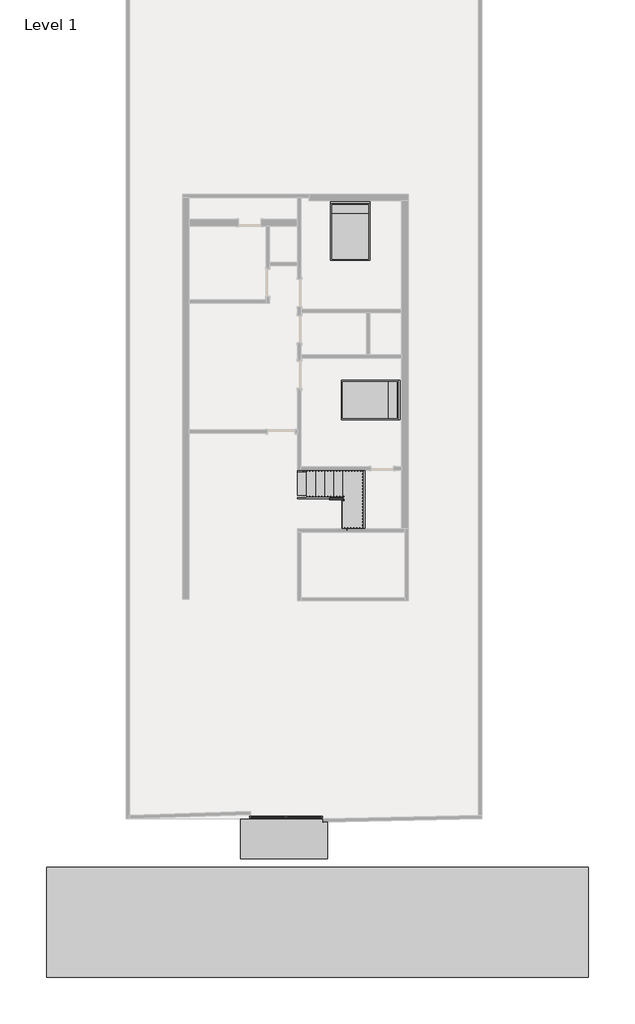
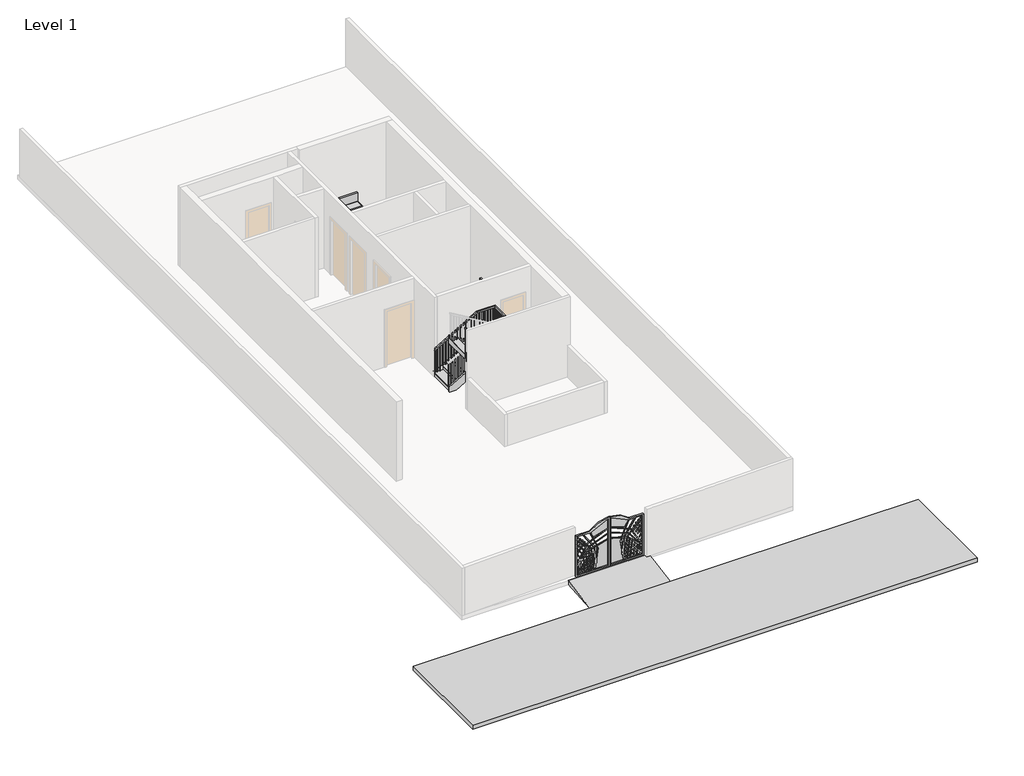
# One storey, part 2 of 2: 6 members, 3 proxies, 2 furniture elements, 1 railing, 1 stair flight.
"""IFC4 building model written with IfcOpenShell, lengths in millimetres."""

from ifc_helpers import new_model, si_unit, frame, origin, place, context, project, spatial, polyline, outline, extrude, faceted_brep, transform, mapped, element, save
from components import generic_models_6bc30956, generic_models_1_generic_models_1_3838245b, generic_models_2_generic_models_2_e98e430d, bed_17739_bed_17739_15c61121, stair_flight_ab8743af

model = new_model("IFC4")

# Units and contexts
model_context = context("Model", 3, world=origin())
ifc_project = project(units=[si_unit("LENGTHUNIT", "METRE", prefix="MILLI")], contexts=[model_context])

# Site, building, storey
site = spatial("IfcSite", under=ifc_project)
building = spatial("IfcBuilding", under=site)
storey = spatial("IfcBuildingStorey", under=building, Name="Level 1", Elevation=0.0)

# Proxies
placement = place(None, origin())
generic_models_shape = generic_models_6bc30956(model_context)
element("IfcBuildingElementProxy", 1, Name="Generic Models", at=placement, inside=storey, context=model_context, shape_type="MappedRepresentation", body=[
    mapped(generic_models_shape, transform((-1579.0915084, -13578.7130462, 0.0), x_axis=(1.0, 0.0, 0.0), y_axis=(0.0, 1.0, 0.0), z_axis=(0.0, 0.0, 1.0))),
])
generic_models_1_generic_models_1_shape = generic_models_1_generic_models_1_3838245b(model_context)
element("IfcBuildingElementProxy", 2, Name="Generic Models 1 : Generic Models 1", ObjectType="Generic Models 1 : Generic Models 1", at=placement, inside=storey, context=model_context, shape_type="MappedRepresentation", body=[
    mapped(generic_models_1_generic_models_1_shape, transform((0.0, 0.0, 0.0), x_axis=(1.0, 0.0, 0.0), y_axis=(0.0, 1.0, 0.0), z_axis=(0.0, 0.0, 1.0))),
])
generic_models_2_generic_models_2_shape = generic_models_2_generic_models_2_e98e430d(model_context)
element("IfcBuildingElementProxy", 3, Name="Generic Models 2 : Generic Models 2", ObjectType="Generic Models 2 : Generic Models 2", at=placement, inside=storey, context=model_context, shape_type="MappedRepresentation", body=[
    mapped(generic_models_2_generic_models_2_shape, transform((0.0, 0.0, 0.0), x_axis=(1.0, 0.0, 0.0), y_axis=(0.0, 1.0, 0.0), z_axis=(0.0, 0.0, 1.0))),
])

# Furniture
bed_17739_bed_17739_shape = bed_17739_bed_17739_15c61121(model_context)
element("IfcFurniture", 4, ObjectType="Bed_17739 : Bed_17739", at=placement, inside=storey, context=model_context, shape_type="MappedRepresentation", body=[
    mapped(bed_17739_bed_17739_shape, transform((592.6084916, 6126.1935985, 0.0), x_axis=(1.0, 0.0, 0.0), y_axis=(0.0, 1.0, 0.0), z_axis=(0.0, 0.0, 1.0))),
])
element("IfcFurniture", 5, ObjectType="Bed_17739 : Bed_17739", at=placement, inside=storey, context=model_context, shape_type="MappedRepresentation", body=[
    mapped(bed_17739_bed_17739_shape, transform((1259.3584916, 455.6435985, 0.0), x_axis=(0.0, -1.0, 0.0), y_axis=(1.0, 0.0, 0.0), z_axis=(0.0, 0.0, 1.0))),
])

# Members
element("IfcMember", 6, ObjectType="Stringer - 2\" Width", at=placement, inside=storey, context=model_context, shape_type="SweptSolid", body=[
    extrude(outline(polyline([(210.4752888, -1179.0415084), (0.0, -1179.0415084), (0.0, -935.6899318), (1151.9647059, 1022.6500682), (1151.9647059, 421.4905007), (210.4752888, -1179.0415084)])), frame((0.0, -1912.9064015, 0.0), z_axis=(0.0, 1.0, 0.0), x_axis=(0.0, 0.0, 1.0)), (0.0, 0.0, 1.0), 50.8),
])
element("IfcMember", 7, ObjectType="Stringer - 2\" Width", at=placement, inside=storey, context=model_context, shape_type="SweptSolid", body=[
    extrude(outline(polyline([(1043.4584916, -1862.1064015), (1094.2584916, -1862.1064015), (1094.2584916, -3894.1064015), (1043.4584916, -3894.1064015), (1043.4584916, -1862.1064015)])), frame((0.0, 0.0, 847.1647059), z_axis=(0.0, 0.0, 1.0), x_axis=(1.0, 0.0, 0.0)), (0.0, 0.0, 1.0), 304.8),
])
element("IfcMember", 8, ObjectType="Stringer - 2\" Width", at=placement, inside=storey, context=model_context, shape_type="SweptSolid", body=[
    extrude(outline(polyline([(847.1647059, 1091.3864826), (2182.7105829, -1179.0415084), (1829.0873079, -1179.0415084), (847.1647059, 490.2269151), (847.1647059, 1091.3864826)])), frame((0.0, -3944.9064015, 0.0), z_axis=(0.0, 1.0, 0.0), x_axis=(0.0, 0.0, 1.0)), (0.0, 0.0, 1.0), 50.8),
])
element("IfcMember", 9, ObjectType="Stringer - 2\" Width", at=placement, inside=storey, context=model_context, shape_type="SweptSolid", body=[
    extrude(outline(polyline([(210.4752888, -1179.0415084), (0.0, -1179.0415084), (0.0, -935.6899318), (723.4402491, 294.1584916), (1077.0635241, 294.1584916), (210.4752888, -1179.0415084)])), frame((0.0, -2878.1064015, 0.0), z_axis=(0.0, 1.0, 0.0), x_axis=(0.0, 0.0, 1.0)), (0.0, 0.0, 1.0), 50.8),
])
element("IfcMember", 10, ObjectType="Stringer - 2\" Width", at=placement, inside=storey, context=model_context, shape_type="SweptSolid", body=[
    extrude(outline(polyline([(294.1584916, -2827.3064015), (344.9584916, -2827.3064015), (344.9584916, -2852.7064015), (294.1584916, -2852.7064015), (294.1584916, -2827.3064015)])), frame((0.0, 0.0, 847.1647059), z_axis=(0.0, 0.0, 1.0), x_axis=(1.0, 0.0, 0.0)), (0.0, 0.0, 1.0), 304.8),
])
element("IfcMember", 11, ObjectType="Stringer - 2\" Width", at=placement, inside=storey, context=model_context, shape_type="SweptSolid", body=[
    extrude(outline(polyline([(932.6167197, 344.9584916), (1286.2399947, 344.9584916), (2182.7105829, -1179.0415084), (1829.0873079, -1179.0415084), (932.6167197, 344.9584916)])), frame((0.0, -2903.5064015, 0.0), z_axis=(0.0, 1.0, 0.0), x_axis=(0.0, 0.0, 1.0)), (0.0, 0.0, 1.0), 50.8),
])

# Railing
element("IfcRailing", 12, ObjectType="Handrail - Rectangular", at=placement, inside=storey, context=model_context, shape_type="SolidModel", body=[
    faceted_brep([(-1179.0415084, -1912.9064015, 1093.6941176), (-1179.0415084, -1912.9064015, 1034.7569051), (-1179.0415084, -1963.7064015, 1034.7569051), (-1179.0415084, -1963.7064015, 1093.6941176), (344.9584916, -1912.9064015, 1990.1647059), (358.7917529, -1912.9064015, 1939.3647059), (358.7917529, -1963.7064015, 1939.3647059), (344.9584916, -1963.7064015, 1990.1647059), (1043.4584916, -1912.9064015, 1990.1647059), (1043.4584916, -1912.9064015, 1939.3647059), (992.6584916, -1963.7064015, 1939.3647059), (992.6584916, -1963.7064015, 1990.1647059), (1043.4584916, -3894.1064015, 1990.1647059), (1043.4584916, -3894.1064015, 1939.3647059), (992.6584916, -3843.3064015, 1939.3647059), (992.6584916, -3843.3064015, 1990.1647059), (649.7584916, -3894.1064015, 1990.1647059), (635.9252304, -3894.1064015, 1939.3647059), (635.9252304, -3843.3064015, 1939.3647059), (649.7584916, -3843.3064015, 1990.1647059), (-1179.0415084, -3894.1064015, 3065.9294118), (-1179.0415084, -3843.3064015, 3065.9294118), (-1179.0415084, -3843.3064015, 3006.9921993), (-1179.0415084, -3894.1064015, 3006.9921993)], [[[0, 1, 2, 3]], [[1, 0, 4, 5]], [[2, 1, 5, 6]], [[3, 2, 6, 7]], [[0, 3, 7, 4]], [[5, 4, 8, 9]], [[6, 5, 9, 10]], [[7, 6, 10, 11]], [[4, 7, 11, 8]], [[9, 8, 12, 13]], [[10, 9, 13, 14]], [[11, 10, 14, 15]], [[8, 11, 15, 12]], [[13, 12, 16, 17]], [[14, 13, 17, 18]], [[15, 14, 18, 19]], [[12, 15, 19, 16]], [[20, 21, 22, 23]], [[17, 16, 20, 23]], [[18, 17, 23, 22]], [[19, 18, 22, 21]], [[16, 19, 21, 20]]]),
    extrude(outline(polyline([(2975.2421993, -1125.0665084), (1972.2352941, -1125.0665084), (1972.2352941, -1106.0165084), (2964.0363169, -1106.0165084), (2975.2421993, -1125.0665084)])), frame((0.0, -3878.2314015, 0.0), z_axis=(0.0, 1.0, 0.0), x_axis=(0.0, 0.0, 1.0)), (0.0, 0.0, 1.0), 19.05),
    extrude(outline(polyline([(2915.4774934, -1023.4665084), (1972.2352941, -1023.4665084), (1972.2352941, -1004.4165084), (2904.271611, -1004.4165084), (2915.4774934, -1023.4665084)])), frame((0.0, -3878.2314015, 0.0), z_axis=(0.0, 1.0, 0.0), x_axis=(0.0, 0.0, 1.0)), (0.0, 0.0, 1.0), 19.05),
    extrude(outline(polyline([(2855.7127875, -921.8665084), (1972.2352941, -921.8665084), (1972.2352941, -902.8165084), (2844.5069051, -902.8165084), (2855.7127875, -921.8665084)])), frame((0.0, -3878.2314015, 0.0), z_axis=(0.0, 1.0, 0.0), x_axis=(0.0, 0.0, 1.0)), (0.0, 0.0, 1.0), 19.05),
    extrude(outline(polyline([(2795.9480816, -820.2665084), (1792.9411765, -820.2665084), (1792.9411765, -801.2165084), (2784.7421993, -801.2165084), (2795.9480816, -820.2665084)])), frame((0.0, -3878.2314015, 0.0), z_axis=(0.0, 1.0, 0.0), x_axis=(0.0, 0.0, 1.0)), (0.0, 0.0, 1.0), 19.05),
    extrude(outline(polyline([(2736.1833757, -718.6665084), (1792.9411765, -718.6665084), (1792.9411765, -699.6165084), (2724.9774934, -699.6165084), (2736.1833757, -718.6665084)])), frame((0.0, -3878.2314015, 0.0), z_axis=(0.0, 1.0, 0.0), x_axis=(0.0, 0.0, 1.0)), (0.0, 0.0, 1.0), 19.05),
    extrude(outline(polyline([(2676.4186699, -617.0665084), (1792.9411765, -617.0665084), (1792.9411765, -598.0165084), (2665.2127875, -598.0165084), (2676.4186699, -617.0665084)])), frame((0.0, -3878.2314015, 0.0), z_axis=(0.0, 1.0, 0.0), x_axis=(0.0, 0.0, 1.0)), (0.0, 0.0, 1.0), 19.05),
    extrude(outline(polyline([(2616.653964, -515.4665084), (1613.6470588, -515.4665084), (1613.6470588, -496.4165084), (2605.4480816, -496.4165084), (2616.653964, -515.4665084)])), frame((0.0, -3878.2314015, 0.0), z_axis=(0.0, 1.0, 0.0), x_axis=(0.0, 0.0, 1.0)), (0.0, 0.0, 1.0), 19.05),
    extrude(outline(polyline([(2556.8892581, -413.8665084), (1613.6470588, -413.8665084), (1613.6470588, -394.8165084), (2545.6833757, -394.8165084), (2556.8892581, -413.8665084)])), frame((0.0, -3878.2314015, 0.0), z_axis=(0.0, 1.0, 0.0), x_axis=(0.0, 0.0, 1.0)), (0.0, 0.0, 1.0), 19.05),
    extrude(outline(polyline([(2497.1245522, -312.2665084), (1613.6470588, -312.2665084), (1613.6470588, -293.2165084), (2485.9186699, -293.2165084), (2497.1245522, -312.2665084)])), frame((0.0, -3878.2314015, 0.0), z_axis=(0.0, 1.0, 0.0), x_axis=(0.0, 0.0, 1.0)), (0.0, 0.0, 1.0), 19.05),
    extrude(outline(polyline([(2437.3598463, -210.6665084), (1434.3529412, -210.6665084), (1434.3529412, -191.6165084), (2426.153964, -191.6165084), (2437.3598463, -210.6665084)])), frame((0.0, -3878.2314015, 0.0), z_axis=(0.0, 1.0, 0.0), x_axis=(0.0, 0.0, 1.0)), (0.0, 0.0, 1.0), 19.05),
    extrude(outline(polyline([(2377.5951404, -109.0665084), (1434.3529412, -109.0665084), (1434.3529412, -90.0165084), (2366.3892581, -90.0165084), (2377.5951404, -109.0665084)])), frame((0.0, -3878.2314015, 0.0), z_axis=(0.0, 1.0, 0.0), x_axis=(0.0, 0.0, 1.0)), (0.0, 0.0, 1.0), 19.05),
    extrude(outline(polyline([(2317.8304346, -7.4665084), (1434.3529412, -7.4665084), (1434.3529412, 11.5834916), (2306.6245522, 11.5834916), (2317.8304346, -7.4665084)])), frame((0.0, -3878.2314015, 0.0), z_axis=(0.0, 1.0, 0.0), x_axis=(0.0, 0.0, 1.0)), (0.0, 0.0, 1.0), 19.05),
    extrude(outline(polyline([(2258.0657287, 94.1334916), (1255.0588235, 94.1334916), (1255.0588235, 113.1834916), (2246.8598463, 113.1834916), (2258.0657287, 94.1334916)])), frame((0.0, -3878.2314015, 0.0), z_axis=(0.0, 1.0, 0.0), x_axis=(0.0, 0.0, 1.0)), (0.0, 0.0, 1.0), 19.05),
    extrude(outline(polyline([(2198.3010228, 195.7334916), (1255.0588235, 195.7334916), (1255.0588235, 214.7834916), (2187.0951404, 214.7834916), (2198.3010228, 195.7334916)])), frame((0.0, -3878.2314015, 0.0), z_axis=(0.0, 1.0, 0.0), x_axis=(0.0, 0.0, 1.0)), (0.0, 0.0, 1.0), 19.05),
    extrude(outline(polyline([(2138.5363169, 297.3334916), (1255.0588235, 297.3334916), (1255.0588235, 316.3834916), (2127.3304346, 316.3834916), (2138.5363169, 297.3334916)])), frame((0.0, -3878.2314015, 0.0), z_axis=(0.0, 1.0, 0.0), x_axis=(0.0, 0.0, 1.0)), (0.0, 0.0, 1.0), 19.05),
    extrude(outline(polyline([(2078.771611, 398.9334916), (1075.7647059, 398.9334916), (1075.7647059, 417.9834916), (2067.5657287, 417.9834916), (2078.771611, 398.9334916)])), frame((0.0, -3878.2314015, 0.0), z_axis=(0.0, 1.0, 0.0), x_axis=(0.0, 0.0, 1.0)), (0.0, 0.0, 1.0), 19.05),
    extrude(outline(polyline([(2019.0069051, 500.5334916), (1075.7647059, 500.5334916), (1075.7647059, 519.5834916), (2007.8010228, 519.5834916), (2019.0069051, 500.5334916)])), frame((0.0, -3878.2314015, 0.0), z_axis=(0.0, 1.0, 0.0), x_axis=(0.0, 0.0, 1.0)), (0.0, 0.0, 1.0), 19.05),
    extrude(outline(polyline([(1959.2421993, 602.1334916), (1075.7647059, 602.1334916), (1075.7647059, 621.1834916), (1948.0363169, 621.1834916), (1959.2421993, 602.1334916)])), frame((0.0, -3878.2314015, 0.0), z_axis=(0.0, 1.0, 0.0), x_axis=(0.0, 0.0, 1.0)), (0.0, 0.0, 1.0), 19.05),
    extrude(outline(polyline([(722.7834916, -3878.2314015), (703.7334916, -3878.2314015), (703.7334916, -3859.1814015), (722.7834916, -3859.1814015), (722.7834916, -3878.2314015)])), frame((0.0, 0.0, 1075.7647059), z_axis=(0.0, 0.0, 1.0), x_axis=(1.0, 0.0, 0.0)), (0.0, 0.0, 1.0), 863.6),
    extrude(outline(polyline([(824.3834916, -3878.2314015), (805.3334916, -3878.2314015), (805.3334916, -3859.1814015), (824.3834916, -3859.1814015), (824.3834916, -3878.2314015)])), frame((0.0, 0.0, 1075.7647059), z_axis=(0.0, 0.0, 1.0), x_axis=(1.0, 0.0, 0.0)), (0.0, 0.0, 1.0), 863.6),
    extrude(outline(polyline([(925.9834916, -3878.2314015), (906.9334916, -3878.2314015), (906.9334916, -3859.1814015), (925.9834916, -3859.1814015), (925.9834916, -3878.2314015)])), frame((0.0, 0.0, 1075.7647059), z_axis=(0.0, 0.0, 1.0), x_axis=(1.0, 0.0, 0.0)), (0.0, 0.0, 1.0), 863.6),
    extrude(outline(polyline([(1027.5834916, -3757.5814015), (1027.5834916, -3776.6314015), (1008.5334916, -3776.6314015), (1008.5334916, -3757.5814015), (1027.5834916, -3757.5814015)])), frame((0.0, 0.0, 1075.7647059), z_axis=(0.0, 0.0, 1.0), x_axis=(1.0, 0.0, 0.0)), (0.0, 0.0, 1.0), 863.6),
    extrude(outline(polyline([(1027.5834916, -3655.9814015), (1027.5834916, -3675.0314015), (1008.5334916, -3675.0314015), (1008.5334916, -3655.9814015), (1027.5834916, -3655.9814015)])), frame((0.0, 0.0, 1075.7647059), z_axis=(0.0, 0.0, 1.0), x_axis=(1.0, 0.0, 0.0)), (0.0, 0.0, 1.0), 863.6),
    extrude(outline(polyline([(1027.5834916, -3554.3814015), (1027.5834916, -3573.4314015), (1008.5334916, -3573.4314015), (1008.5334916, -3554.3814015), (1027.5834916, -3554.3814015)])), frame((0.0, 0.0, 1075.7647059), z_axis=(0.0, 0.0, 1.0), x_axis=(1.0, 0.0, 0.0)), (0.0, 0.0, 1.0), 863.6),
    extrude(outline(polyline([(1027.5834916, -3452.7814015), (1027.5834916, -3471.8314015), (1008.5334916, -3471.8314015), (1008.5334916, -3452.7814015), (1027.5834916, -3452.7814015)])), frame((0.0, 0.0, 1075.7647059), z_axis=(0.0, 0.0, 1.0), x_axis=(1.0, 0.0, 0.0)), (0.0, 0.0, 1.0), 863.6),
    extrude(outline(polyline([(1027.5834916, -3351.1814015), (1027.5834916, -3370.2314015), (1008.5334916, -3370.2314015), (1008.5334916, -3351.1814015), (1027.5834916, -3351.1814015)])), frame((0.0, 0.0, 1075.7647059), z_axis=(0.0, 0.0, 1.0), x_axis=(1.0, 0.0, 0.0)), (0.0, 0.0, 1.0), 863.6),
    extrude(outline(polyline([(1027.5834916, -3249.5814015), (1027.5834916, -3268.6314015), (1008.5334916, -3268.6314015), (1008.5334916, -3249.5814015), (1027.5834916, -3249.5814015)])), frame((0.0, 0.0, 1075.7647059), z_axis=(0.0, 0.0, 1.0), x_axis=(1.0, 0.0, 0.0)), (0.0, 0.0, 1.0), 863.6),
    extrude(outline(polyline([(1027.5834916, -3147.9814015), (1027.5834916, -3167.0314015), (1008.5334916, -3167.0314015), (1008.5334916, -3147.9814015), (1027.5834916, -3147.9814015)])), frame((0.0, 0.0, 1075.7647059), z_axis=(0.0, 0.0, 1.0), x_axis=(1.0, 0.0, 0.0)), (0.0, 0.0, 1.0), 863.6),
    extrude(outline(polyline([(1027.5834916, -3046.3814015), (1027.5834916, -3065.4314015), (1008.5334916, -3065.4314015), (1008.5334916, -3046.3814015), (1027.5834916, -3046.3814015)])), frame((0.0, 0.0, 1075.7647059), z_axis=(0.0, 0.0, 1.0), x_axis=(1.0, 0.0, 0.0)), (0.0, 0.0, 1.0), 863.6),
    extrude(outline(polyline([(1027.5834916, -2944.7814015), (1027.5834916, -2963.8314015), (1008.5334916, -2963.8314015), (1008.5334916, -2944.7814015), (1027.5834916, -2944.7814015)])), frame((0.0, 0.0, 1075.7647059), z_axis=(0.0, 0.0, 1.0), x_axis=(1.0, 0.0, 0.0)), (0.0, 0.0, 1.0), 863.6),
    extrude(outline(polyline([(1027.5834916, -2843.1814015), (1027.5834916, -2862.2314015), (1008.5334916, -2862.2314015), (1008.5334916, -2843.1814015), (1027.5834916, -2843.1814015)])), frame((0.0, 0.0, 1075.7647059), z_axis=(0.0, 0.0, 1.0), x_axis=(1.0, 0.0, 0.0)), (0.0, 0.0, 1.0), 863.6),
    extrude(outline(polyline([(1027.5834916, -2741.5814015), (1027.5834916, -2760.6314015), (1008.5334916, -2760.6314015), (1008.5334916, -2741.5814015), (1027.5834916, -2741.5814015)])), frame((0.0, 0.0, 1075.7647059), z_axis=(0.0, 0.0, 1.0), x_axis=(1.0, 0.0, 0.0)), (0.0, 0.0, 1.0), 863.6),
    extrude(outline(polyline([(1027.5834916, -2639.9814015), (1027.5834916, -2659.0314015), (1008.5334916, -2659.0314015), (1008.5334916, -2639.9814015), (1027.5834916, -2639.9814015)])), frame((0.0, 0.0, 1075.7647059), z_axis=(0.0, 0.0, 1.0), x_axis=(1.0, 0.0, 0.0)), (0.0, 0.0, 1.0), 863.6),
    extrude(outline(polyline([(1027.5834916, -2538.3814015), (1027.5834916, -2557.4314015), (1008.5334916, -2557.4314015), (1008.5334916, -2538.3814015), (1027.5834916, -2538.3814015)])), frame((0.0, 0.0, 1075.7647059), z_axis=(0.0, 0.0, 1.0), x_axis=(1.0, 0.0, 0.0)), (0.0, 0.0, 1.0), 863.6),
    extrude(outline(polyline([(1027.5834916, -2436.7814015), (1027.5834916, -2455.8314015), (1008.5334916, -2455.8314015), (1008.5334916, -2436.7814015), (1027.5834916, -2436.7814015)])), frame((0.0, 0.0, 1075.7647059), z_axis=(0.0, 0.0, 1.0), x_axis=(1.0, 0.0, 0.0)), (0.0, 0.0, 1.0), 863.6),
    extrude(outline(polyline([(1027.5834916, -2335.1814015), (1027.5834916, -2354.2314015), (1008.5334916, -2354.2314015), (1008.5334916, -2335.1814015), (1027.5834916, -2335.1814015)])), frame((0.0, 0.0, 1075.7647059), z_axis=(0.0, 0.0, 1.0), x_axis=(1.0, 0.0, 0.0)), (0.0, 0.0, 1.0), 863.6),
    extrude(outline(polyline([(1027.5834916, -2233.5814015), (1027.5834916, -2252.6314015), (1008.5334916, -2252.6314015), (1008.5334916, -2233.5814015), (1027.5834916, -2233.5814015)])), frame((0.0, 0.0, 1075.7647059), z_axis=(0.0, 0.0, 1.0), x_axis=(1.0, 0.0, 0.0)), (0.0, 0.0, 1.0), 863.6),
    extrude(outline(polyline([(1027.5834916, -2131.9814015), (1027.5834916, -2151.0314015), (1008.5334916, -2151.0314015), (1008.5334916, -2131.9814015), (1027.5834916, -2131.9814015)])), frame((0.0, 0.0, 1075.7647059), z_axis=(0.0, 0.0, 1.0), x_axis=(1.0, 0.0, 0.0)), (0.0, 0.0, 1.0), 863.6),
    extrude(outline(polyline([(1027.5834916, -2030.3814015), (1027.5834916, -2049.4314015), (1008.5334916, -2049.4314015), (1008.5334916, -2030.3814015), (1027.5834916, -2030.3814015)])), frame((0.0, 0.0, 1075.7647059), z_axis=(0.0, 0.0, 1.0), x_axis=(1.0, 0.0, 0.0)), (0.0, 0.0, 1.0), 863.6),
    extrude(outline(polyline([(945.0334916, -1928.7814015), (964.0834916, -1928.7814015), (964.0834916, -1947.8314015), (945.0334916, -1947.8314015), (945.0334916, -1928.7814015)])), frame((0.0, 0.0, 1075.7647059), z_axis=(0.0, 0.0, 1.0), x_axis=(1.0, 0.0, 0.0)), (0.0, 0.0, 1.0), 863.6),
    extrude(outline(polyline([(843.4334916, -1928.7814015), (862.4834916, -1928.7814015), (862.4834916, -1947.8314015), (843.4334916, -1947.8314015), (843.4334916, -1928.7814015)])), frame((0.0, 0.0, 1075.7647059), z_axis=(0.0, 0.0, 1.0), x_axis=(1.0, 0.0, 0.0)), (0.0, 0.0, 1.0), 863.6),
    extrude(outline(polyline([(741.8334916, -1928.7814015), (760.8834916, -1928.7814015), (760.8834916, -1947.8314015), (741.8334916, -1947.8314015), (741.8334916, -1928.7814015)])), frame((0.0, 0.0, 1075.7647059), z_axis=(0.0, 0.0, 1.0), x_axis=(1.0, 0.0, 0.0)), (0.0, 0.0, 1.0), 863.6),
    extrude(outline(polyline([(640.2334916, -1928.7814015), (659.2834916, -1928.7814015), (659.2834916, -1947.8314015), (640.2334916, -1947.8314015), (640.2334916, -1928.7814015)])), frame((0.0, 0.0, 1075.7647059), z_axis=(0.0, 0.0, 1.0), x_axis=(1.0, 0.0, 0.0)), (0.0, 0.0, 1.0), 863.6),
    extrude(outline(polyline([(538.6334916, -1928.7814015), (557.6834916, -1928.7814015), (557.6834916, -1947.8314015), (538.6334916, -1947.8314015), (538.6334916, -1928.7814015)])), frame((0.0, 0.0, 1075.7647059), z_axis=(0.0, 0.0, 1.0), x_axis=(1.0, 0.0, 0.0)), (0.0, 0.0, 1.0), 863.6),
    extrude(outline(polyline([(437.0334916, -1928.7814015), (456.0834916, -1928.7814015), (456.0834916, -1947.8314015), (437.0334916, -1947.8314015), (437.0334916, -1928.7814015)])), frame((0.0, 0.0, 1075.7647059), z_axis=(0.0, 0.0, 1.0), x_axis=(1.0, 0.0, 0.0)), (0.0, 0.0, 1.0), 863.6),
    extrude(outline(polyline([(1925.6245522, 335.4334916), (1075.7647059, 335.4334916), (1075.7647059, 354.4834916), (1936.8304346, 354.4834916), (1925.6245522, 335.4334916)])), frame((0.0, -1947.8314015, 0.0), z_axis=(0.0, 1.0, 0.0), x_axis=(0.0, 0.0, 1.0)), (0.0, 0.0, 1.0), 19.05),
    extrude(outline(polyline([(1865.8598463, 233.8334916), (896.4705882, 233.8334916), (896.4705882, 252.8834916), (1877.0657287, 252.8834916), (1865.8598463, 233.8334916)])), frame((0.0, -1947.8314015, 0.0), z_axis=(0.0, 1.0, 0.0), x_axis=(0.0, 0.0, 1.0)), (0.0, 0.0, 1.0), 19.05),
    extrude(outline(polyline([(1806.0951404, 132.2334916), (896.4705882, 132.2334916), (896.4705882, 151.2834916), (1817.3010228, 151.2834916), (1806.0951404, 132.2334916)])), frame((0.0, -1947.8314015, 0.0), z_axis=(0.0, 1.0, 0.0), x_axis=(0.0, 0.0, 1.0)), (0.0, 0.0, 1.0), 19.05),
    extrude(outline(polyline([(1746.3304346, 30.6334916), (896.4705882, 30.6334916), (896.4705882, 49.6834916), (1757.5363169, 49.6834916), (1746.3304346, 30.6334916)])), frame((0.0, -1947.8314015, 0.0), z_axis=(0.0, 1.0, 0.0), x_axis=(0.0, 0.0, 1.0)), (0.0, 0.0, 1.0), 19.05),
    extrude(outline(polyline([(1686.5657287, -70.9665084), (717.1764706, -70.9665084), (717.1764706, -51.9165084), (1697.771611, -51.9165084), (1686.5657287, -70.9665084)])), frame((0.0, -1947.8314015, 0.0), z_axis=(0.0, 1.0, 0.0), x_axis=(0.0, 0.0, 1.0)), (0.0, 0.0, 1.0), 19.05),
    extrude(outline(polyline([(1626.8010228, -172.5665084), (717.1764706, -172.5665084), (717.1764706, -153.5165084), (1638.0069051, -153.5165084), (1626.8010228, -172.5665084)])), frame((0.0, -1947.8314015, 0.0), z_axis=(0.0, 1.0, 0.0), x_axis=(0.0, 0.0, 1.0)), (0.0, 0.0, 1.0), 19.05),
    extrude(outline(polyline([(1567.0363169, -274.1665084), (717.1764706, -274.1665084), (717.1764706, -255.1165084), (1578.2421993, -255.1165084), (1567.0363169, -274.1665084)])), frame((0.0, -1947.8314015, 0.0), z_axis=(0.0, 1.0, 0.0), x_axis=(0.0, 0.0, 1.0)), (0.0, 0.0, 1.0), 19.05),
    extrude(outline(polyline([(1507.271611, -375.7665084), (537.8823529, -375.7665084), (537.8823529, -356.7165084), (1518.4774934, -356.7165084), (1507.271611, -375.7665084)])), frame((0.0, -1947.8314015, 0.0), z_axis=(0.0, 1.0, 0.0), x_axis=(0.0, 0.0, 1.0)), (0.0, 0.0, 1.0), 19.05),
    extrude(outline(polyline([(1447.5069051, -477.3665084), (537.8823529, -477.3665084), (537.8823529, -458.3165084), (1458.7127875, -458.3165084), (1447.5069051, -477.3665084)])), frame((0.0, -1947.8314015, 0.0), z_axis=(0.0, 1.0, 0.0), x_axis=(0.0, 0.0, 1.0)), (0.0, 0.0, 1.0), 19.05),
    extrude(outline(polyline([(1387.7421993, -578.9665084), (537.8823529, -578.9665084), (537.8823529, -559.9165084), (1398.9480816, -559.9165084), (1387.7421993, -578.9665084)])), frame((0.0, -1947.8314015, 0.0), z_axis=(0.0, 1.0, 0.0), x_axis=(0.0, 0.0, 1.0)), (0.0, 0.0, 1.0), 19.05),
    extrude(outline(polyline([(1327.9774934, -680.5665084), (358.5882353, -680.5665084), (358.5882353, -661.5165084), (1339.1833757, -661.5165084), (1327.9774934, -680.5665084)])), frame((0.0, -1947.8314015, 0.0), z_axis=(0.0, 1.0, 0.0), x_axis=(0.0, 0.0, 1.0)), (0.0, 0.0, 1.0), 19.05),
    extrude(outline(polyline([(1268.2127875, -782.1665084), (358.5882353, -782.1665084), (358.5882353, -763.1165084), (1279.4186699, -763.1165084), (1268.2127875, -782.1665084)])), frame((0.0, -1947.8314015, 0.0), z_axis=(0.0, 1.0, 0.0), x_axis=(0.0, 0.0, 1.0)), (0.0, 0.0, 1.0), 19.05),
    extrude(outline(polyline([(1208.4480816, -883.7665084), (358.5882353, -883.7665084), (358.5882353, -864.7165084), (1219.653964, -864.7165084), (1208.4480816, -883.7665084)])), frame((0.0, -1947.8314015, 0.0), z_axis=(0.0, 1.0, 0.0), x_axis=(0.0, 0.0, 1.0)), (0.0, 0.0, 1.0), 19.05),
    extrude(outline(polyline([(1148.6833757, -985.3665084), (179.2941176, -985.3665084), (179.2941176, -966.3165084), (1159.8892581, -966.3165084), (1148.6833757, -985.3665084)])), frame((0.0, -1947.8314015, 0.0), z_axis=(0.0, 1.0, 0.0), x_axis=(0.0, 0.0, 1.0)), (0.0, 0.0, 1.0), 19.05),
    extrude(outline(polyline([(1088.9186699, -1086.9665084), (179.2941176, -1086.9665084), (179.2941176, -1067.9165084), (1100.1245522, -1067.9165084), (1088.9186699, -1086.9665084)])), frame((0.0, -1947.8314015, 0.0), z_axis=(0.0, 1.0, 0.0), x_axis=(0.0, 0.0, 1.0)), (0.0, 0.0, 1.0), 19.05),
    extrude(outline(polyline([(1027.5834916, -3859.1814015), (1027.5834916, -3878.2314015), (1008.5334916, -3878.2314015), (1008.5334916, -3859.1814015), (1027.5834916, -3859.1814015)])), frame((0.0, 0.0, 1075.7647059), z_axis=(0.0, 0.0, 1.0), x_axis=(1.0, 0.0, 0.0)), (0.0, 0.0, 1.0), 863.6),
    extrude(outline(polyline([(1008.5334916, -1928.7814015), (1027.5834916, -1928.7814015), (1027.5834916, -1947.8314015), (1008.5334916, -1947.8314015), (1008.5334916, -1928.7814015)])), frame((0.0, 0.0, 1075.7647059), z_axis=(0.0, 0.0, 1.0), x_axis=(1.0, 0.0, 0.0)), (0.0, 0.0, 1.0), 863.6),
    extrude(outline(polyline([(3006.9921993, -1179.0415084), (1972.2352941, -1179.0415084), (1972.2352941, -1159.9915084), (2995.7863169, -1159.9915084), (3006.9921993, -1179.0415084)])), frame((0.0, -3878.2314015, 0.0), z_axis=(0.0, 1.0, 0.0), x_axis=(0.0, 0.0, 1.0)), (0.0, 0.0, 1.0), 19.05),
    extrude(outline(polyline([(1034.7569051, -1179.0415084), (179.2941176, -1179.0415084), (179.2941176, -1159.9915084), (1045.9627875, -1159.9915084), (1034.7569051, -1179.0415084)])), frame((0.0, -1947.8314015, 0.0), z_axis=(0.0, 1.0, 0.0), x_axis=(0.0, 0.0, 1.0)), (0.0, 0.0, 1.0), 19.05),
])

# Stair flight
stair_flight_shape = stair_flight_ab8743af(model_context)
element("IfcStairFlight", 13, ObjectType="2\" Tread 1\" Nosing 1/4\" Riser", at=placement, inside=storey, context=model_context, shape_type="MappedRepresentation", body=[
    mapped(stair_flight_shape, transform((0.0, 0.0, 0.0), x_axis=(1.0, 0.0, 0.0), y_axis=(0.0, 1.0, 0.0), z_axis=(0.0, 0.0, 1.0))),
])

save(model, "model.ifc")

# Revit data of these elements
# Type
#   m.s. sheet = none
#   2" x2" pipe = none
#   1"x1"pipe = none
#   Default Elevation = 0
# Type "Bed_17739 : Bed_17739"
#   Default Elevation = 0
# Type "Handrail - Rectangular"
#   Assembly Code = "C2010400"
#   built-in parameter 1008612 = 0.0416667 (stored number, unit not read)
#   built-in parameter 1008611 = 0.0416667 (stored number, unit not read)
#   built-in parameter 1008609 = 0.333333 (stored number, unit not read)
#   built-in parameter 1008604 = 0.166667 (stored number, unit not read)
#   built-in parameter 1008603 = 0.166667 (stored number, unit not read)
#   Railing Height = 3' - 0"
#   built-in parameter 1008630 = 2
#   built-in parameter 1008610 = 2
#   built-in parameter 1008618 = Baluster - Square : 3/4"
# Element 1 (IfcBuildingElementProxy)
#   Phase Created = New Construction
#   Materials on its faces: "r1"
# Element 2 (IfcBuildingElementProxy, "Generic Models 1 : Generic Models 1")
#   Phase Created = New Construction
# Element 3 (IfcBuildingElementProxy, "Generic Models 2 : Generic Models 2")
#   Phase Created = New Construction
# Elements 4, 5 (IfcFurniture, "Bed_17739 : Bed_17739")
#   Phase Created = New Construction
#   Materials on its faces: "legs", "sheets", "bed frame", "Blanket"
# Elements 6, 7, 8, 9, 10, 11 (IfcMember, "Stringer - 2\" Width")
#   Phase Created = New Construction
# Element 12 (IfcRailing, "Handrail - Rectangular")
#   Phase Created = New Construction
# Element 13 (IfcStairFlight, "2\" Tread 1\" Nosing 1/4\" Riser")
#   Phase Created = New Construction
# Materials
#   "r1": class "Generic", colour RGB 120 120 120, transparency 0, Cost = 0
#   "legs": colour RGB 90 73 37, transparency 0, Cost = 0
#   "sheets": colour RGB 200 195 176, transparency 0, Cost = 0
#   "bed frame": colour RGB 90 73 37, transparency 0, Cost = 0
#   "Blanket": class "System", colour RGB 59 0 1, transparency 0, Cost = 0
